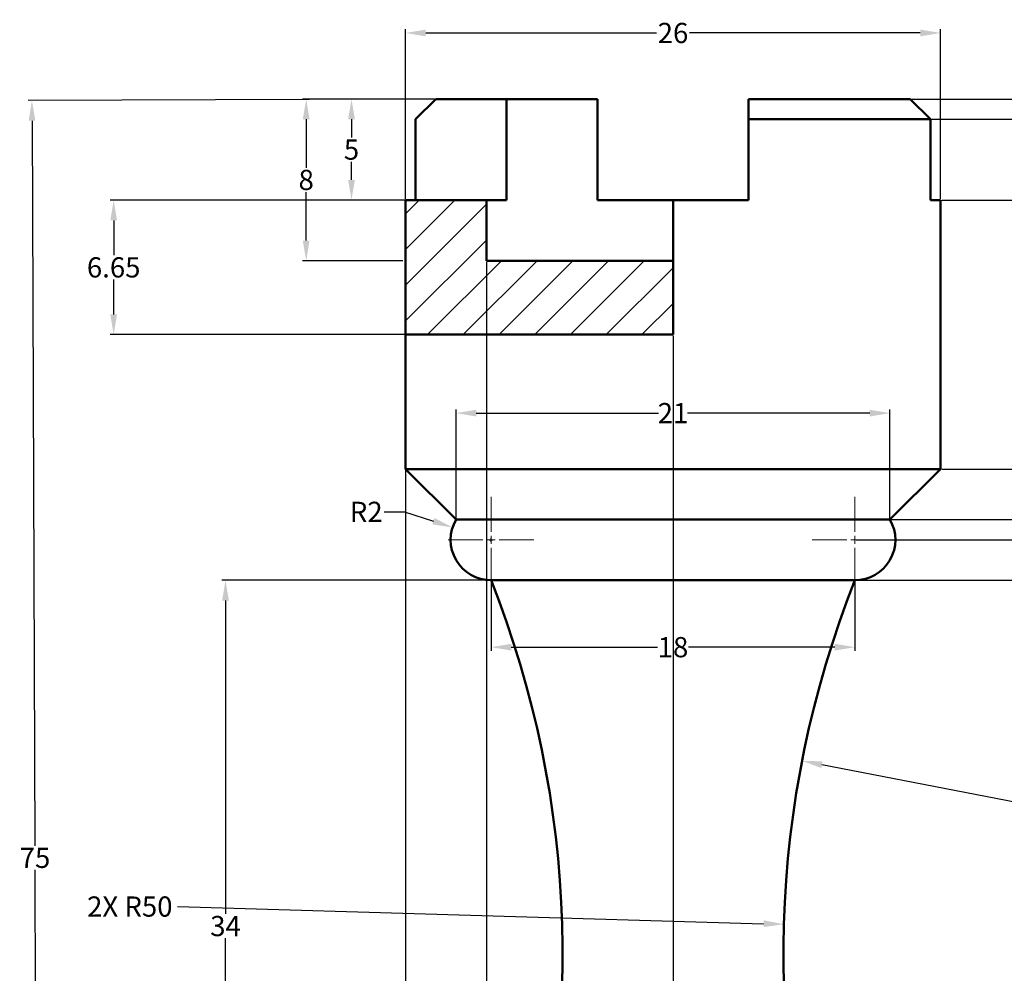
# Model space of a CAD drawing. Units: millimetres. Extents: x 31 to 232, y 35 to 192.
# Tile 2 of 5: x 31 to 80, y 75 to 122. Entities that reach past the tile are written whole.
import ezdxf

# ---------------------------------------------------------------- set-up
doc = ezdxf.new("R2010")
doc.units = ezdxf.units.MM
doc.header["$MEASUREMENT"] = 0
doc.linetypes.add('CENTER', pattern=[50.8, 31.75, -6.35, 6.35, -6.35])
for name, color, linetype, lineweight in [('M-CNTR', 1, 'CENTER', 18), ('M-DIMS', 2, 'Continuous', 25), ('M-HATC', 8, 'Continuous', 18), ('M-OUTL', 7, 'Continuous', 50)]:
    doc.layers.add(name, color=color, linetype=linetype, lineweight=lineweight)
doc.styles.get("Standard").update_dxf_attribs({"font": 'arial.ttf'})
doc.dimstyles.get("Standard").update_dxf_attribs({"dimtxt": 1, "dimasz": 1, "dimexe": 0.18, "dimexo": 0.0625, "dimgap": 0.09, "dimtad": 0, "dimtih": 1, "dimtoh": 1, "dimdec": 0, "dimzin": 0, "dimdsep": 46, "dimtxsty": 'Standard', "dimcen": 0.09, "dimadec": 0, "dimazin": 0, "dimtfac": 1, "dimtdec": 0, "dimtofl": 0, "dimtmove": 0, "dimatfit": 3, "dimfxl": 1, "dimtolj": 1, "dimtzin": 0, "dimarcsym": 0})

# ---------------------------------------------------------------- blocks, each defined once
blk = doc.blocks.new('*D10')
at = {"layer": 'Defpoints', "color": 0, "transparency": 16777216}
for p in [(119.236, 75.81), (119.423, 75.81), (71.774, 60.083)]:
    blk.add_point(p, dxfattribs=at)
at = {"layer": 'M-DIMS', "color": 0, "lineweight": -2, "transparency": 16777216}
for p, q in [((119.298, 75.81), (119.603, 75.81)), ((119.423, 74.81), (119.423, 68.547)), ((119.423, 61.083), (119.423, 67.346)), ((71.836, 60.083), (119.603, 60.083))]:
    blk.add_line(p, q, dxfattribs=at)
at = {"layer": 'M-DIMS', "color": 0, "transparency": 16777216}
for points in [[(119.256, 74.81), (119.589, 74.81), (119.423, 75.81)], [(119.256, 61.083), (119.589, 61.083), (119.423, 60.083)]]:
    blk.add_solid(points, dxfattribs=at)
at = {"layer": 'M-DIMS', "color": 0, "transparency": 16777216, "insert": (119.423, 67.946), "char_height": 1, "attachment_point": 5}
blk.add_mtext('\\A1;16', dxfattribs=at)
blk = doc.blocks.new('*D11')
at = {"layer": 'Defpoints', "color": 0, "transparency": 16777216}
for p in [(72.774, 94.283), (119.423, 94.283), (119.236, 75.81)]:
    blk.add_point(p, dxfattribs=at)
at = {"layer": 'M-DIMS', "color": 0, "lineweight": -2, "transparency": 16777216}
for p, q in [((72.836, 94.283), (119.603, 94.283)), ((119.423, 93.283), (119.423, 85.647)), ((119.423, 76.81), (119.423, 84.446)), ((119.298, 75.81), (119.603, 75.81))]:
    blk.add_line(p, q, dxfattribs=at)
at = {"layer": 'M-DIMS', "color": 0, "transparency": 16777216}
for points in [[(119.256, 93.283), (119.589, 93.283), (119.423, 94.283)], [(119.256, 76.81), (119.589, 76.81), (119.423, 75.81)]]:
    blk.add_solid(points, dxfattribs=at)
at = {"layer": 'M-DIMS', "color": 0, "transparency": 16777216, "insert": (119.423, 85.046), "char_height": 1, "attachment_point": 5}
blk.add_mtext('\\A1;18', dxfattribs=at)
blk = doc.blocks.new('*D12')
at = {"layer": 'Defpoints', "color": 0, "transparency": 16777216}
for p in [(72.774, 96.283), (118.478, 96.283), (72.774, 94.283)]:
    blk.add_point(p, dxfattribs=at)
at = {"layer": 'M-DIMS', "color": 0, "lineweight": -2, "transparency": 16777216}
for p, q in [((118.478, 97.283), (118.478, 98.283)), ((72.836, 96.283), (118.658, 96.283)), ((72.836, 94.283), (118.658, 94.283)), ((118.478, 93.283), (118.478, 92.283))]:
    blk.add_line(p, q, dxfattribs=at)
at = {"layer": 'M-DIMS', "color": 0, "transparency": 16777216}
for points in [[(118.312, 97.283), (118.645, 97.283), (118.478, 96.283)], [(118.312, 93.283), (118.645, 93.283), (118.478, 94.283)]]:
    blk.add_solid(points, dxfattribs=at)
at = {"layer": 'M-DIMS', "color": 0, "transparency": 16777216, "insert": (118.478, 95.283), "char_height": 1, "attachment_point": 5}
blk.add_mtext('\\A1;2', dxfattribs=at)
blk = doc.blocks.new('*D13')
at = {"layer": 'Defpoints', "color": 0, "transparency": 16777216}
for p in [(74.506, 97.283), (120.627, 97.283), (72.774, 96.283)]:
    blk.add_point(p, dxfattribs=at)
at = {"layer": 'M-DIMS', "color": 0, "lineweight": -2, "transparency": 16777216}
for p, q in [((120.627, 98.283), (120.627, 99.283)), ((120.627, 99.283), (121.627, 99.283)), ((74.568, 97.283), (120.807, 97.283)), ((72.836, 96.283), (120.807, 96.283)), ((120.627, 95.283), (120.627, 94.283))]:
    blk.add_line(p, q, dxfattribs=at)
at = {"layer": 'M-DIMS', "color": 0, "transparency": 16777216}
for points in [[(120.46, 98.283), (120.794, 98.283), (120.627, 97.283)], [(120.46, 95.283), (120.794, 95.283), (120.627, 96.283)]]:
    blk.add_solid(points, dxfattribs=at)
at = {"layer": 'M-DIMS', "color": 0, "transparency": 16777216, "insert": (121.901, 99.283), "char_height": 1, "attachment_point": 5}
blk.add_mtext('\\A1;1', dxfattribs=at)
blk = doc.blocks.new('*D14')
at = {"layer": 'Defpoints', "color": 0, "transparency": 16777216}
for p in [(77.006, 99.783), (116.013, 99.783), (74.506, 97.283)]:
    blk.add_point(p, dxfattribs=at)
at = {"layer": 'M-DIMS', "color": 0, "lineweight": -2, "transparency": 16777216}
for p, q in [((116.013, 99.783), (116.013, 100.783)), ((116.013, 100.783), (117.013, 100.783)), ((77.068, 99.783), (116.193, 99.783)), ((116.013, 98.283), (116.013, 98.783)), ((74.568, 97.283), (116.193, 97.283))]:
    blk.add_line(p, q, dxfattribs=at)
at = {"layer": 'M-DIMS', "color": 0, "transparency": 16777216}
for points in [[(115.846, 98.783), (116.18, 98.783), (116.013, 99.783)], [(115.846, 98.283), (116.18, 98.283), (116.013, 97.283)]]:
    blk.add_solid(points, dxfattribs=at)
at = {"layer": 'M-DIMS', "color": 0, "transparency": 16777216, "insert": (117.43, 100.783), "char_height": 1, "attachment_point": 5}
blk.add_mtext('\\A1;3', dxfattribs=at)
blk = doc.blocks.new('*D15')
at = {"layer": 'Defpoints', "color": 0, "transparency": 16777216}
for p in [(77.006, 113.083), (119.423, 113.083), (77.006, 99.783)]:
    blk.add_point(p, dxfattribs=at)
at = {"layer": 'M-DIMS', "color": 0, "lineweight": -2, "transparency": 16777216}
for p, q in [((77.068, 113.083), (119.603, 113.083)), ((119.423, 112.083), (119.423, 107.034)), ((119.423, 100.783), (119.423, 105.832)), ((77.068, 99.783), (119.603, 99.783))]:
    blk.add_line(p, q, dxfattribs=at)
at = {"layer": 'M-DIMS', "color": 0, "transparency": 16777216}
for points in [[(119.256, 112.083), (119.589, 112.083), (119.423, 113.083)], [(119.256, 100.783), (119.589, 100.783), (119.423, 99.783)]]:
    blk.add_solid(points, dxfattribs=at)
at = {"layer": 'M-DIMS', "color": 0, "transparency": 16777216, "insert": (119.423, 106.433), "char_height": 1, "attachment_point": 5}
blk.add_mtext('\\A1;13', dxfattribs=at)
blk = doc.blocks.new('*D16')
at = {"layer": 'Defpoints', "color": 0, "transparency": 16777216}
for p in [(76.506, 117.083), (119.892, 117.083), (77.006, 113.083)]:
    blk.add_point(p, dxfattribs=at)
at = {"layer": 'M-DIMS', "color": 0, "lineweight": -2, "transparency": 16777216}
for p, q in [((119.892, 117.083), (119.892, 118.083)), ((119.892, 118.083), (120.892, 118.083)), ((76.568, 117.083), (120.072, 117.083)), ((119.892, 114.083), (119.892, 116.083)), ((77.068, 113.083), (120.072, 113.083))]:
    blk.add_line(p, q, dxfattribs=at)
at = {"layer": 'M-DIMS', "color": 0, "transparency": 16777216}
for points in [[(119.726, 116.083), (120.059, 116.083), (119.892, 117.083)], [(119.726, 114.083), (120.059, 114.083), (119.892, 113.083)]]:
    blk.add_solid(points, dxfattribs=at)
at = {"layer": 'M-DIMS', "color": 0, "transparency": 16777216, "insert": (121.328, 118.083), "char_height": 1, "attachment_point": 5}
blk.add_mtext('\\A1;4', dxfattribs=at)
blk = doc.blocks.new('*D17')
at = {"layer": 'Defpoints', "color": 0, "transparency": 16777216}
for p in [(75.506, 118.083), (115.962, 118.083), (76.506, 117.083)]:
    blk.add_point(p, dxfattribs=at)
at = {"layer": 'M-DIMS', "color": 0, "lineweight": -2, "transparency": 16777216}
for p, q in [((115.962, 119.083), (115.962, 120.083)), ((115.962, 120.083), (116.962, 120.083)), ((75.568, 118.083), (116.142, 118.083)), ((76.568, 117.083), (116.142, 117.083)), ((115.962, 116.083), (115.962, 115.083))]:
    blk.add_line(p, q, dxfattribs=at)
at = {"layer": 'M-DIMS', "color": 0, "transparency": 16777216}
for points in [[(115.795, 119.083), (116.128, 119.083), (115.962, 118.083)], [(115.795, 116.083), (116.128, 116.083), (115.962, 117.083)]]:
    blk.add_solid(points, dxfattribs=at)
at = {"layer": 'M-DIMS', "color": 0, "transparency": 16777216, "insert": (117.236, 120.083), "char_height": 1, "attachment_point": 5}
blk.add_mtext('\\A1;1', dxfattribs=at)
blk = doc.blocks.new('*D23')
at = {"layer": 'Defpoints', "color": 0, "transparency": 16777216}
for p in [(70.155, 85.355), (119.236, 75.81)]:
    blk.add_point(p, dxfattribs=at)
at = {"layer": 'M-DIMS', "color": 0, "lineweight": -2, "transparency": 16777216}
blk.add_line((86.946, 82.089), (71.137, 85.164), dxfattribs=at)
at = {"layer": 'M-DIMS', "color": 0, "transparency": 16777216}
blk.add_solid([(71.169, 85.328), (71.105, 85), (70.155, 85.355)], dxfattribs=at)
at = {"layer": 'M-DIMS', "color": 0, "transparency": 16777216, "insert": (88.229, 82.089), "char_height": 1, "attachment_point": 5}
blk.add_mtext('\\A1;R50', dxfattribs=at)
blk = doc.blocks.new('*D24')
at = {"layer": 'Defpoints', "color": 0, "transparency": 16777216}
for p in [(32.062, 118.008), (50.471, 118.083), (50.774, 43.183)]:
    blk.add_point(p, dxfattribs=at)
at = {"layer": 'M-DIMS', "color": 0, "lineweight": -2, "transparency": 16777216}
for p, q in [((50.408, 118.083), (31.882, 118.008)), ((32.066, 117.008), (32.211, 81.157)), ((32.361, 44.108), (32.216, 79.96)), ((50.711, 43.183), (32.185, 43.108))]:
    blk.add_line(p, q, dxfattribs=at)
at = {"layer": 'M-DIMS', "color": 0, "transparency": 16777216}
for points in [[(32.233, 117.009), (31.9, 117.008), (32.062, 118.008)], [(32.528, 44.109), (32.195, 44.108), (32.365, 43.108)]]:
    blk.add_solid(points, dxfattribs=at)
at = {"layer": 'M-DIMS', "color": 0, "transparency": 16777216, "insert": (32.214, 80.558), "char_height": 1, "attachment_point": 5}
blk.add_mtext('\\A1;75', dxfattribs=at)
blk = doc.blocks.new('*D25')
at = {"layer": 'Defpoints', "color": 0, "transparency": 16777216}
for p in [(52.042, 118.083), (47.87, 113.083), (52.042, 113.083)]:
    blk.add_point(p, dxfattribs=at)
at = {"layer": 'M-DIMS', "color": 0, "lineweight": -2, "transparency": 16777216}
for p, q in [((51.979, 118.083), (47.69, 118.083)), ((47.87, 117.083), (47.87, 116.181)), ((47.87, 114.083), (47.87, 114.984)), ((51.979, 113.083), (47.69, 113.083))]:
    blk.add_line(p, q, dxfattribs=at)
at = {"layer": 'M-DIMS', "color": 0, "transparency": 16777216}
for points in [[(47.704, 117.083), (48.037, 117.083), (47.87, 118.083)], [(47.704, 114.083), (48.037, 114.083), (47.87, 113.083)]]:
    blk.add_solid(points, dxfattribs=at)
at = {"layer": 'M-DIMS', "color": 0, "transparency": 16777216, "insert": (47.87, 115.583), "char_height": 1, "attachment_point": 5}
blk.add_mtext('\\A1;5', dxfattribs=at)
blk = doc.blocks.new('*D26')
at = {"layer": 'Defpoints', "color": 0, "transparency": 16777216}
for p in [(50.471, 118.083), (45.629, 110.083), (50.471, 110.083)]:
    blk.add_point(p, dxfattribs=at)
at = {"layer": 'M-DIMS', "color": 0, "lineweight": -2, "transparency": 16777216}
for p, q in [((50.408, 118.083), (45.449, 118.083)), ((45.629, 117.083), (45.629, 114.683)), ((45.629, 111.083), (45.629, 113.482)), ((50.408, 110.083), (45.449, 110.083))]:
    blk.add_line(p, q, dxfattribs=at)
at = {"layer": 'M-DIMS', "color": 0, "transparency": 16777216}
for points in [[(45.463, 117.083), (45.796, 117.083), (45.629, 118.083)], [(45.463, 111.083), (45.796, 111.083), (45.629, 110.083)]]:
    blk.add_solid(points, dxfattribs=at)
at = {"layer": 'M-DIMS', "color": 0, "transparency": 16777216, "insert": (45.629, 114.083), "char_height": 1, "attachment_point": 5}
blk.add_mtext('\\A1;8', dxfattribs=at)
blk = doc.blocks.new('*D27')
at = {"layer": 'Defpoints', "color": 0, "transparency": 16777216}
for p in [(77.006, 121.351), (50.542, 113.083), (77.006, 113.083)]:
    blk.add_point(p, dxfattribs=at)
at = {"layer": 'M-DIMS', "color": 0, "lineweight": -2, "transparency": 16777216}
for p, q in [((50.542, 113.145), (50.542, 121.531)), ((51.542, 121.351), (62.959, 121.351)), ((76.006, 121.351), (64.588, 121.351)), ((77.006, 113.145), (77.006, 121.531))]:
    blk.add_line(p, q, dxfattribs=at)
at = {"layer": 'M-DIMS', "color": 0, "transparency": 16777216}
for points in [[(51.542, 121.518), (51.542, 121.184), (50.542, 121.351)], [(76.006, 121.518), (76.006, 121.184), (77.006, 121.351)]]:
    blk.add_solid(points, dxfattribs=at)
at = {"layer": 'M-DIMS', "color": 0, "transparency": 16777216, "insert": (63.774, 121.351), "char_height": 1, "attachment_point": 5}
blk.add_mtext('\\A1;26', dxfattribs=at)
blk = doc.blocks.new('*D28')
at = {"layer": 'Defpoints', "color": 0, "transparency": 16777216}
for p in [(74.506, 102.55), (53.042, 97.283), (74.506, 97.283)]:
    blk.add_point(p, dxfattribs=at)
at = {"layer": 'M-DIMS', "color": 0, "lineweight": -2, "transparency": 16777216}
for p, q in [((53.042, 97.345), (53.042, 102.73)), ((54.042, 102.55), (63.055, 102.55)), ((73.506, 102.55), (64.492, 102.55)), ((74.506, 97.345), (74.506, 102.73))]:
    blk.add_line(p, q, dxfattribs=at)
at = {"layer": 'M-DIMS', "color": 0, "transparency": 16777216}
for points in [[(54.042, 102.716), (54.042, 102.383), (53.042, 102.55)], [(73.506, 102.716), (73.506, 102.383), (74.506, 102.55)]]:
    blk.add_solid(points, dxfattribs=at)
at = {"layer": 'M-DIMS', "color": 0, "transparency": 16777216, "insert": (63.774, 102.55), "char_height": 1, "attachment_point": 5}
blk.add_mtext('\\A1;21', dxfattribs=at)
blk = doc.blocks.new('*D29')
at = {"layer": 'Defpoints', "color": 0, "transparency": 16777216}
for p in [(54.774, 94.283), (72.774, 94.283), (72.774, 90.975)]:
    blk.add_point(p, dxfattribs=at)
at = {"layer": 'M-DIMS', "color": 0, "lineweight": -2, "transparency": 16777216}
for p, q in [((54.774, 94.22), (54.774, 90.795)), ((72.774, 94.22), (72.774, 90.795)), ((55.774, 90.975), (63.013, 90.975)), ((71.774, 90.975), (64.534, 90.975))]:
    blk.add_line(p, q, dxfattribs=at)
at = {"layer": 'M-DIMS', "color": 0, "transparency": 16777216}
for points in [[(55.774, 91.142), (55.774, 90.809), (54.774, 90.975)], [(71.774, 91.142), (71.774, 90.809), (72.774, 90.975)]]:
    blk.add_solid(points, dxfattribs=at)
at = {"layer": 'M-DIMS', "color": 0, "transparency": 16777216, "insert": (63.774, 90.975), "char_height": 1, "attachment_point": 5}
blk.add_mtext('\\A1;18', dxfattribs=at)
blk = doc.blocks.new('*D30')
at = {"layer": 'Defpoints', "color": 0, "transparency": 16777216}
for p in [(41.638, 94.283), (63.774, 94.283), (63.774, 60.083)]:
    blk.add_point(p, dxfattribs=at)
at = {"layer": 'M-DIMS', "color": 0, "lineweight": -2, "transparency": 16777216}
for p, q in [((63.711, 94.283), (41.458, 94.283)), ((41.638, 93.283), (41.638, 77.784)), ((41.638, 61.083), (41.638, 76.582)), ((63.711, 60.083), (41.458, 60.083))]:
    blk.add_line(p, q, dxfattribs=at)
at = {"layer": 'M-DIMS', "color": 0, "transparency": 16777216}
for points in [[(41.471, 93.283), (41.805, 93.283), (41.638, 94.283)], [(41.471, 61.083), (41.805, 61.083), (41.638, 60.083)]]:
    blk.add_solid(points, dxfattribs=at)
at = {"layer": 'M-DIMS', "color": 0, "transparency": 16777216, "insert": (41.638, 77.183), "char_height": 1, "attachment_point": 5}
blk.add_mtext('\\A1;34', dxfattribs=at)
blk = doc.blocks.new('*D31')
at = {"layer": 'Defpoints', "color": 0, "transparency": 16777216}
for p in [(52.87, 96.898), (54.774, 96.283)]:
    blk.add_point(p, dxfattribs=at)
at = {"layer": 'M-DIMS', "color": 0, "lineweight": -2, "transparency": 16777216}
for p, q in [((49.491, 97.667), (50.491, 97.667)), ((50.491, 97.667), (51.919, 97.205)), ((54.684, 96.283), (54.864, 96.283)), ((54.774, 96.193), (54.774, 96.373))]:
    blk.add_line(p, q, dxfattribs=at)
at = {"layer": 'M-DIMS', "color": 0, "transparency": 16777216}
blk.add_solid([(51.97, 97.364), (51.868, 97.047), (52.87, 96.898)], dxfattribs=at)
at = {"layer": 'M-DIMS', "color": 0, "transparency": 16777216, "insert": (48.599, 97.667), "char_height": 1, "attachment_point": 5}
blk.add_mtext('\\A1;R2', dxfattribs=at)
blk = doc.blocks.new('*U33')
at = {"layer": 'M-CNTR', "color": 0, "transparency": 16777216}
for p, q in [((0, 0.4), (0, 2.12)), ((-2.12, 0), (-0.4, 0)), ((0.4, 0), (2.12, 0)), ((0, -2.12), (0, -0.4))]:
    blk.add_line(p, q, dxfattribs=at)
at = {"layer": 'M-CNTR', "color": 0, "linetype": 'Continuous', "transparency": 16777216}
for p, q in [((-0.2, 0), (0.2, 0)), ((0, -0.2), (0, 0.2))]:
    blk.add_line(p, q, dxfattribs=at)
blk = doc.blocks.new('*U34')
at = {"layer": 'M-CNTR', "color": 0, "transparency": 16777216}
for p, q in [((0, 0.4), (0, 2.12)), ((-2.12, 0), (-0.4, 0)), ((0.4, 0), (2.12, 0)), ((0, -2.12), (0, -0.4))]:
    blk.add_line(p, q, dxfattribs=at)
at = {"layer": 'M-CNTR', "color": 0, "linetype": 'Continuous', "transparency": 16777216}
for p, q in [((-0.2, 0), (0.2, 0)), ((0, -0.2), (0, 0.2))]:
    blk.add_line(p, q, dxfattribs=at)
blk = doc.blocks.new('*D42')
at = {"layer": 'Defpoints', "color": 0, "transparency": 16777216}
for p in [(50.542, 113.083), (36.106, 106.433), (50.542, 106.433)]:
    blk.add_point(p, dxfattribs=at)
at = {"layer": 'M-DIMS', "color": 0, "lineweight": -2, "transparency": 16777216}
for p, q in [((50.479, 113.083), (35.926, 113.083)), ((36.106, 112.083), (36.106, 110.358)), ((36.106, 107.433), (36.106, 109.157)), ((50.479, 106.433), (35.926, 106.433))]:
    blk.add_line(p, q, dxfattribs=at)
at = {"layer": 'M-DIMS', "color": 0, "transparency": 16777216}
for points in [[(35.939, 112.083), (36.273, 112.083), (36.106, 113.083)], [(35.939, 107.433), (36.273, 107.433), (36.106, 106.433)]]:
    blk.add_solid(points, dxfattribs=at)
at = {"layer": 'M-DIMS', "color": 0, "transparency": 16777216, "insert": (36.106, 109.758), "char_height": 1, "attachment_point": 5}
blk.add_mtext('\\A1;6.65', dxfattribs=at)
blk = doc.blocks.new('*D43')
at = {"layer": 'Defpoints', "color": 0, "transparency": 16777216}
for p in [(50.542, 106.433), (63.774, 106.433), (63.774, 35.333)]:
    blk.add_point(p, dxfattribs=at)
at = {"layer": 'M-DIMS', "color": 0, "lineweight": -2, "transparency": 16777216}
for p, q in [((50.542, 106.37), (50.542, 35.153)), ((63.774, 106.37), (63.774, 35.153)), ((51.542, 35.333), (55.044, 35.333)), ((62.774, 35.333), (59.271, 35.333))]:
    blk.add_line(p, q, dxfattribs=at)
at = {"layer": 'M-DIMS', "color": 0, "transparency": 16777216}
for points in [[(51.542, 35.5), (51.542, 35.166), (50.542, 35.333)], [(62.774, 35.5), (62.774, 35.166), (63.774, 35.333)]]:
    blk.add_solid(points, dxfattribs=at)
at = {"layer": 'M-DIMS', "color": 0, "transparency": 16777216, "insert": (57.158, 35.333), "char_height": 1, "attachment_point": 5}
blk.add_mtext('\\A1;13.232', dxfattribs=at)
blk = doc.blocks.new('*D44')
at = {"layer": 'Defpoints', "color": 0, "transparency": 16777216}
for p in [(50.542, 113.083), (54.542, 110.083), (54.542, 35.333)]:
    blk.add_point(p, dxfattribs=at)
at = {"layer": 'M-DIMS', "color": 0, "lineweight": -2, "transparency": 16777216}
for p, q in [((50.542, 113.02), (50.542, 35.153)), ((54.542, 110.02), (54.542, 35.153)), ((51.542, 35.333), (52.106, 35.333)), ((53.542, 35.333), (52.977, 35.333))]:
    blk.add_line(p, q, dxfattribs=at)
at = {"layer": 'M-DIMS', "color": 0, "transparency": 16777216}
for points in [[(51.542, 35.5), (51.542, 35.166), (50.542, 35.333)], [(53.542, 35.5), (53.542, 35.166), (54.542, 35.333)]]:
    blk.add_solid(points, dxfattribs=at)
at = {"layer": 'M-DIMS', "color": 0, "transparency": 16777216, "insert": (52.542, 35.333), "char_height": 1, "attachment_point": 5}
blk.add_mtext('\\A1;4', dxfattribs=at)
blk = doc.blocks.new('*D48')
at = {"layer": 'Defpoints', "color": 0, "transparency": 16777216}
for p in [(69.257, 77.271), (119.236, 75.81)]:
    blk.add_point(p, dxfattribs=at)
at = {"layer": 'M-DIMS', "color": 0, "lineweight": -2, "transparency": 16777216}
for p, q in [((39.27, 78.148), (68.258, 77.3)), ((119.146, 75.81), (119.326, 75.81)), ((119.236, 75.72), (119.236, 75.9))]:
    blk.add_line(p, q, dxfattribs=at)
at = {"layer": 'M-DIMS', "color": 0, "transparency": 16777216}
blk.add_solid([(68.263, 77.467), (68.253, 77.134), (69.257, 77.271)], dxfattribs=at)
at = {"layer": 'M-DIMS', "color": 0, "transparency": 16777216, "insert": (36.904, 78.148), "char_height": 1, "attachment_point": 5}
blk.add_mtext('\\A1;2X R50', dxfattribs=at)

msp = doc.modelspace()

# ---------------------------------------------------------------- hatches: boundary and pattern name
at = {"layer": 'M-HATC'}
h = msp.add_hatch(dxfattribs=at)
h.set_pattern_fill('ANSI31', color=256, scale=10)
h.paths.add_polyline_path([(63.7736, 110.0829), (54.5416, 110.0829), (54.5416, 113.0829), (50.5416, 113.0829), (50.5416, 106.4329), (63.7736, 106.4329)])

# ---------------------------------------------------------------- linework, layer by layer
at = {"layer": 'M-OUTL'}
for p, q in [((51.0416, 117.0829), (52.0416, 118.0829)), ((52.0416, 118.0829), (60.0416, 118.0829)), ((55.5416, 113.0829), (55.5416, 118.0829)), ((60.0416, 118.0829), (60.0416, 113.0829)), ((75.5057, 118.0829), (67.5057, 118.0829)), ((67.5057, 118.0829), (67.5057, 113.0829)), ((76.5057, 117.0829), (75.5057, 118.0829)), ((51.0416, 113.0829), (51.0416, 117.0829)), ((76.5057, 117.0829), (67.5057, 117.0829)), ((76.5057, 113.0829), (76.5057, 117.0829)), ((50.5416, 99.7829), (50.5416, 113.0829)), ((50.5416, 113.0829), (54.5416, 113.0829)), ((50.5416, 113.0829), (51.0416, 113.0829)), ((50.5416, 113.0829), (50.5416, 99.7829)), ((50.5416, 113.0829), (54.5416, 113.0829)), ((54.5416, 113.0829), (54.5416, 110.0829)), ((54.5416, 113.0829), (55.5416, 113.0829)), ((60.0416, 113.0829), (63.7736, 113.0829)), ((67.5057, 113.0829), (63.7736, 113.0829)), ((63.7736, 110.0829), (63.7736, 113.0829)), ((77.0057, 113.0829), (76.5057, 113.0829)), ((77.0057, 113.0829), (76.5057, 113.0829)), ((77.0057, 113.0829), (76.5057, 113.0829)), ((77.0057, 99.7829), (77.0057, 113.0829)), ((77.0057, 113.0829), (77.0057, 99.7829)), ((54.5416, 110.0829), (63.7736, 110.0829)), ((63.7736, 110.0829), (63.7736, 106.4329)), ((63.7736, 110.0829), (63.7736, 106.4329)), ((50.5416, 106.4329), (63.7736, 106.4329)), ((53.0416, 97.2829), (50.5416, 99.7829)), ((50.5416, 99.7829), (63.7736, 99.7829)), ((77.0057, 99.7829), (63.7736, 99.7829)), ((74.5057, 97.2829), (77.0057, 99.7829)), ((53.0416, 97.2829), (62.0416, 97.2829)), ((62.0416, 97.2829), (63.7736, 97.2829)), ((65.5057, 97.2829), (63.7736, 97.2829)), ((74.5057, 97.2829), (65.5057, 97.2829)), ((63.7736, 94.2829), (54.7736, 94.2829)), ((63.7736, 94.2829), (72.7736, 94.2829))]:
    msp.add_line(p, q, dxfattribs=at)
for centre, radius, start, end in [((54.7736, 96.2829), 2, 150, 270), ((72.7736, 96.2829), 2, 270, 30), ((8.3113, 75.8097), 50, 341.66715, 21.68252), ((119.2359, 75.8097), 50, 158.31748, 198.33285)]:
    msp.add_arc(centre, radius, start, end, dxfattribs=at)

# ---------------------------------------------------------------- block references
at = {"layer": 'M-CNTR'}
for name, p in [('*U34', (54.7736, 96.2829)), ('*U33', (72.7736, 96.2829))]:
    msp.add_blockref(name, p, dxfattribs=at)

# ---------------------------------------------------------------- dimensions: what is measured, and where the dimension line sits
at = {"layer": 'M-DIMS'}
for base, p1, p2, override, picture, middle in [((77.0057, 121.3509), (50.5416, 113.0829), (77.0057, 113.0829), {"dimclrd": 0, "dimclre": 0, "dimclrt": 0}, '*D27', (63.7736, 121.3509)), ((54.5416, 35.3329), (50.5416, 113.0829), (54.5416, 110.0829), {"dimdec": 0, "dimlfac": 1, "dimrnd": 0, "dimzin": 0, "dimdsep": 46, "dimlunit": 2}, '*D44', (52.5416, 35.3329)), ((63.7736, 35.3329), (50.5416, 106.4329), (63.7736, 106.4329), {"dimdec": 3, "dimlfac": 1, "dimrnd": 0, "dimzin": 0, "dimdsep": 46, "dimlunit": 2}, '*D43', (57.1576, 35.3329)), ((74.5057, 102.5495), (53.0416, 97.2829), (74.5057, 97.2829), {"dimclrd": 0, "dimclre": 0, "dimclrt": 0}, '*D28', (63.7736, 102.5495)), ((72.7736, 90.9754), (54.7736, 94.2829), (72.7736, 94.2829), {"dimclrd": 0, "dimclre": 0, "dimclrt": 0}, '*D29', (63.7736, 90.9754))]:
    dim = msp.add_linear_dim(base=base, p1=p1, p2=p2, dimstyle='Standard', override=override, dxfattribs=at)
    dim.commit()
    dim.dimension.update_dxf_attribs({"geometry": picture, "text_midpoint": middle})
for base, p1, p2, picture, middle in [((115.9616, 118.0829), (76.5057, 117.0829), (75.5057, 118.0829), '*D17', (117.2358, 120.0829)), ((119.8924, 117.0829), (77.0057, 113.0829), (76.5057, 117.0829), '*D16', (121.3282, 118.0829)), ((118.4782, 96.2829), (72.7736, 94.2829), (72.7736, 96.2829), '*D12', (118.4782, 95.2829))]:
    dim = msp.add_linear_dim(base=base, p1=p1, p2=p2, angle=270, dimstyle='Standard', override={"dimclrd": 0, "dimclre": 0, "dimclrt": 0}, dxfattribs=at)
    dim.commit()
    dim.dimension.update_dxf_attribs({"geometry": picture, "text_midpoint": middle, "dimtype": 160})
dim = msp.add_aligned_dim(p1=(50.7736, 43.1829), p2=(50.4706, 118.0829), distance=18.4084, dimstyle='Standard', override={"dimclrd": 0, "dimclre": 0, "dimclrt": 0}, dxfattribs=at)
dim.commit()
dim.dimension.update_dxf_attribs({"geometry": '*D24', "text_midpoint": (32.2138, 80.5584)})
for base, p1, p2, angle, override, picture, middle in [((45.6292, 110.0829), (50.4706, 118.0829), (50.4706, 110.0829), 90, {"dimclrd": 0, "dimclre": 0, "dimclrt": 0}, '*D26', (45.6292, 114.0829)), ((47.8703, 113.0829), (52.0416, 118.0829), (52.0416, 113.0829), 90, {"dimclrd": 0, "dimclre": 0, "dimclrt": 0}, '*D25', (47.8703, 115.5829)), ((36.106, 106.4329), (50.5416, 113.0829), (50.5416, 106.4329), 90, {"dimdec": 2, "dimlfac": 1, "dimrnd": 0, "dimzin": 0, "dimdsep": 46, "dimlunit": 2}, '*D42', (36.106, 109.7579)), ((119.4225, 113.0829), (77.0057, 99.7829), (77.0057, 113.0829), 270, {"dimclrd": 0, "dimclre": 0, "dimclrt": 0}, '*D15', (119.4225, 106.4329)), ((116.0129246117, 99.7828853826), (74.5056541686, 97.2828853826), (77.0056541686, 99.7828853826), 270, {"dimclrd": 0, "dimclre": 0, "dimclrt": 0}, '*D14', (117.4303461669, 100.7828853826)), ((120.6271, 97.2829), (72.7736, 96.2829), (74.5057, 97.2829), 270, {"dimclrd": 0, "dimclre": 0, "dimclrt": 0}, '*D13', (121.9012, 99.2829)), ((41.6381, 94.2829), (63.7736, 60.0829), (63.7736, 94.2829), 90, {"dimclrd": 0, "dimclre": 0, "dimclrt": 0}, '*D30', (41.6381, 77.1829)), ((119.4225, 94.2829), (119.2359, 75.8097), (72.7736, 94.2829), 270, {"dimclrd": 0, "dimclre": 0, "dimclrt": 0}, '*D11', (119.4225, 85.0463)), ((119.4225, 75.8097), (71.7736, 60.0829), (119.2359, 75.8097), 270, {"dimclrd": 0, "dimclre": 0, "dimclrt": 0}, '*D10', (119.4225, 67.9463))]:
    dim = msp.add_linear_dim(base=base, p1=p1, p2=p2, angle=angle, dimstyle='Standard', override=override, dxfattribs=at)
    dim.commit()
    dim.dimension.update_dxf_attribs({"geometry": picture, "text_midpoint": middle})
for center, mpoint, picture, middle in [((54.7736, 96.2829), (52.8705, 96.8978), '*D31', (48.5994, 97.6666)), ((119.2359, 75.8097), (70.1554, 85.3549), '*D23', (86.9462, 82.0894))]:
    dim = msp.add_radius_dim(center=center, mpoint=mpoint, dimstyle='Standard', override={"dimclrd": 0, "dimclre": 0, "dimclrt": 0}, dxfattribs=at)
    dim.commit()
    dim.dimension.update_dxf_attribs({"geometry": picture, "text_midpoint": middle, "dimtype": 164})
dim = msp.add_radius_dim(center=(119.2359, 75.8097), mpoint=(69.2572, 77.271), text='2X <>', dimstyle='Standard', override={"dimdec": 0, "dimlfac": 1, "dimrnd": 0, "dimzin": 0, "dimdsep": 46, "dimlunit": 2}, dxfattribs=at)
dim.commit()
dim.dimension.update_dxf_attribs({"geometry": '*D48', "text_midpoint": (39.27, 78.1478), "dimtype": 164})

doc.saveas('drawing.dxf')
